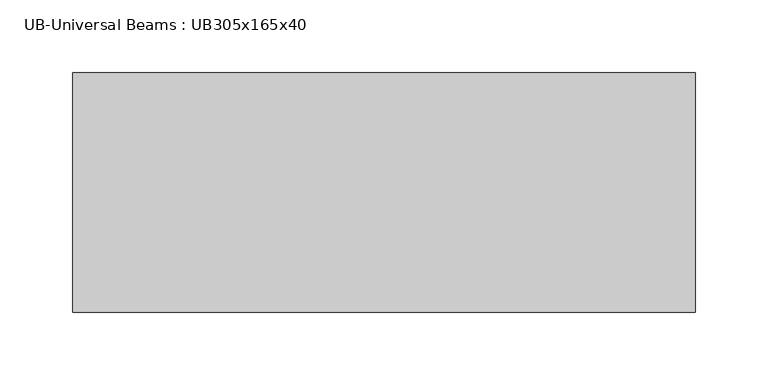
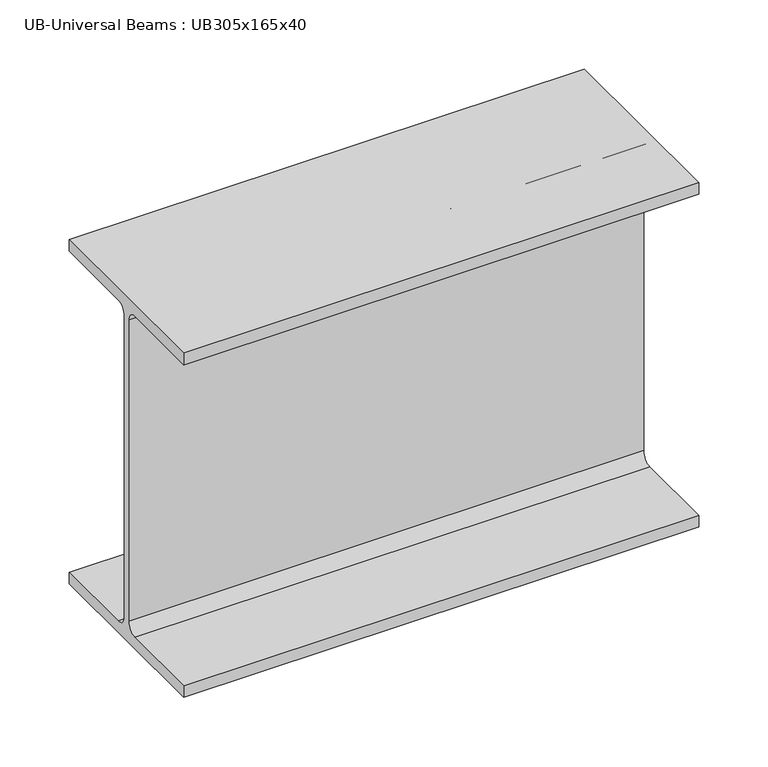
"""IFC4 building model written with IfcOpenShell, lengths in millimetres: beam geometry, UB-Universal Beams : UB305x165x40."""

from ifc_helpers import new_model, si_unit, point, frame, frame_2d, origin, place, context, project, spatial, polyline, circle_curve, trimmed, segment, composite_curve, outline, extrude, source, transform, mapped, element, save


def ub_universal_beams_ub305x165x40_890a58b8(model_context):
    return source(origin(), model_context, "Body", "SweptSolid", [
        extrude(outline(composite_curve([segment(polyline([(-82.5, -141.5), (-11.9, -141.5)]), True, "CONTINUOUS"), segment(trimmed(circle_curve(frame_2d((-11.9, -132.6)), 8.9), [point((-11.9, -141.5))], [point((-3.0, -132.6))], True, "CARTESIAN"), True, "CONTINUOUS"), segment(polyline([(-3.0, -132.6), (-3.0, 132.6)]), True, "CONTINUOUS"), segment(trimmed(circle_curve(frame_2d((-11.9, 132.6)), 8.9), [point((-3.0, 132.6))], [point((-11.9, 141.5))], True, "CARTESIAN"), True, "CONTINUOUS"), segment(polyline([(-11.9, 141.5), (-82.5, 141.5), (-82.5, 151.7), (82.5, 151.7), (82.5, 141.5), (11.9, 141.5)]), True, "CONTINUOUS"), segment(trimmed(circle_curve(frame_2d((11.9, 132.6)), 8.9), [point((11.9, 141.5))], [point((3.0, 132.6))], True, "CARTESIAN"), True, "CONTINUOUS"), segment(polyline([(3.0, 132.6), (3.0, -132.6)]), True, "CONTINUOUS"), segment(trimmed(circle_curve(frame_2d((11.9, -132.6)), 8.9), [point((3.0, -132.6))], [point((11.9, -141.5))], True, "CARTESIAN"), True, "CONTINUOUS"), segment(polyline([(11.9, -141.5), (82.5, -141.5), (82.5, -151.7), (-82.5, -151.7), (-82.5, -141.5)]), True, "CONTINUOUS")], self_intersect=False)), frame((-797.5, 0.0, 0.0), z_axis=(1.0, 0.0, 0.0), x_axis=(0.0, 1.0, 0.0)), (0.0, 0.0, 1.0), 429.1),
    ])


if __name__ == "__main__":
    model = new_model("IFC4")
    model_context = context("Model", 3, world=origin())
    ifc_project = project(units=[si_unit("LENGTHUNIT", "METRE", prefix="MILLI")], contexts=[model_context])
    site = spatial("IfcSite", under=ifc_project)
    building = spatial("IfcBuilding", under=site)
    placement = place(None, origin())
    ub_universal_beams_ub305x165x40_shape = ub_universal_beams_ub305x165x40_890a58b8(model_context)
    element("IfcBeam", 1, ObjectType="UB-Universal Beams : UB305x165x40", at=placement, inside=building, context=model_context, shape_type="MappedRepresentation", body=[
        mapped(ub_universal_beams_ub305x165x40_shape, transform((0.0, 0.0, 0.0), x_axis=(1.0, 0.0, 0.0), y_axis=(0.0, 1.0, 0.0), z_axis=(0.0, 0.0, 1.0))),
    ])
    save(model, "model.ifc")

# Revit data of these elements
# Type "UB-Universal Beams : UB305x165x40"
#   Section Name Key = "UB305X165X40"
#   Width = 16.5 cm
#   Web Thickness = 0.6 cm
#   Web Fillet = 0.89 cm
#   Warping Constant = 164000.0 cm⁶
#   Torsional Moment of Inertia = 14.70 cm⁴
#   Section Area = 51.3 cm²
#   Plastic Modulus weak axis = 142.0 cm³
#   Plastic Modulus strong axis = 623.0 cm³
#   Nominal Weight = 40.2999 kgf/m
#   Moment of Inertia weak axis = 764.00 cm⁴
#   Moment of Inertia strong axis = 8503.00 cm⁴
#   Height = 30.34 cm
#   Flange Thickness = 1.02 cm
#   Elastic Modulus weak axis = 92.6 cm³
#   Elastic Modulus strong axis = 560.0 cm³
#   Centroid Vertical = 15.17 cm
#   Centroid Horizontal = 8.25 cm
#   Bolt Spacing = 9.0 cm
#   Length [instance default] = 1500 mm
#   Structural Material [instance default] = Metal - Steel 43-275
#   Type Comments = ""
#   Assembly Code = ""
# Element 1 (IfcBeam, "UB-Universal Beams : UB305x165x40")
#   Materials on its faces: "Metal - Steel 43-275"
# Materials
#   "Metal - Steel 43-275": class "Metal", colour RGB 247 247 247, transparency 0, Cost = 0
